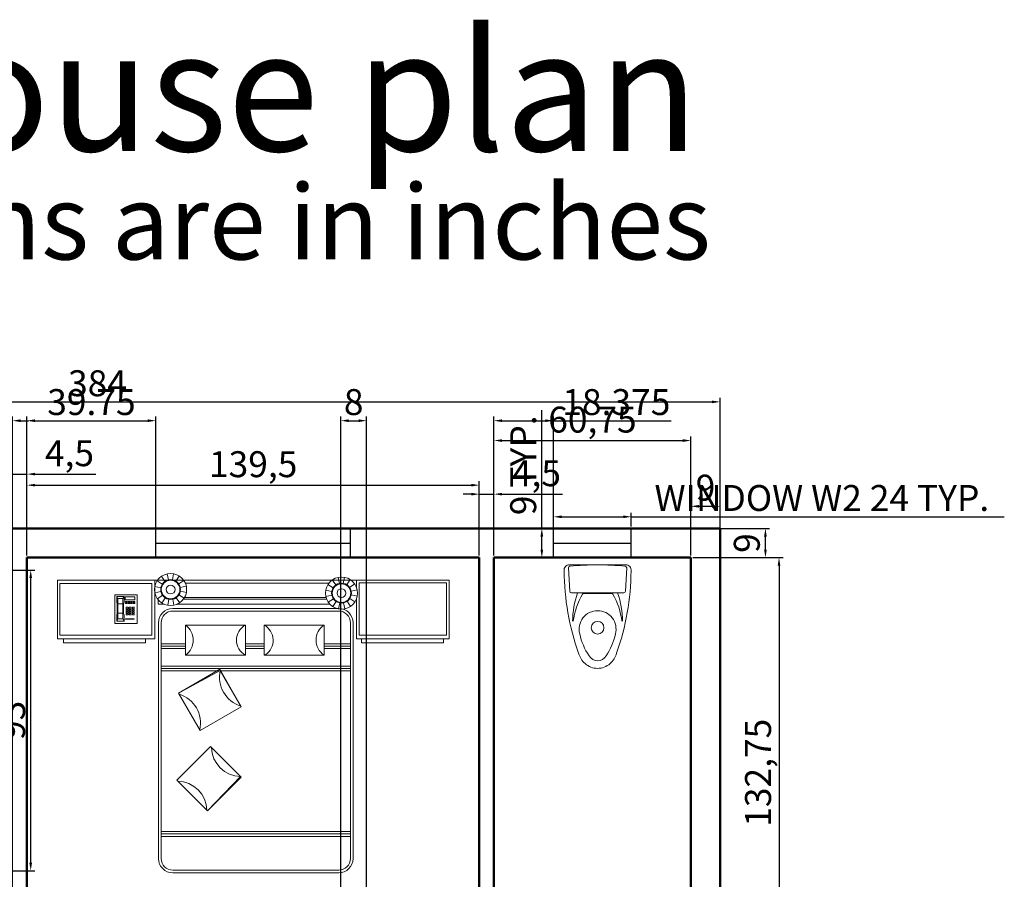
# Model space of a CAD drawing. Units: inches. Extents: x -349 to 9053, y 635 to 6001.
# Tile 6 of 7: x 498 to 802, y 1018 to 1283. Entities that reach past the tile are written whole.
import ezdxf

# ---------------------------------------------------------------- set-up
doc = ezdxf.new("R2010")
doc.units = ezdxf.units.IN
for name, color, linetype, lineweight in [('A-ANNO-DIMS', 2, 'Continuous', 18), ('A-ANNO-TEXT', 7, 'Continuous', 25), ('A-FLOR-FIXT', 7, 'Continuous', 18), ('A-FURN', 8, 'Continuous', 18), ('A-GLAZ', 4, 'Continuous', 25), ('A-WALL', 7, 'Continuous', 50)]:
    doc.layers.add(name, color=color, linetype=linetype, lineweight=lineweight)
doc.styles.get("Standard").update_dxf_attribs({"font": 'arial.ttf'})
doc.dimstyles.new('ISO-25', dxfattribs={"dimtxt": 8, "dimasz": 2.5, "dimexe": 1.25, "dimexo": 0.625, "dimtad": 1, "dimtxsty": 'Standard', "dimcen": 2.5, "dimadec": 0, "dimazin": 0, "dimtfac": 1, "dimtmove": 0, "dimatfit": 3, "dimfxl": 1, "dimarcsym": 0})

# ---------------------------------------------------------------- blocks, each defined once
blk = doc.blocks.new('A$C18EB7ED0')
for p, q in [((0.7653, 2.1814), (0.7911, 2.1442)), ((0.8076, 2.1998), (0.8172, 2.1555)), ((0.8537, 2.2006), (0.8456, 2.1559)), ((0.8966, 2.1836), (0.8721, 2.1455)), ((2.0643, 2.1733), (2.0739, 2.129)), ((2.1105, 2.1741), (2.1024, 2.1295)), ((0, 2.1539), (2.8801, 2.1539)), ((0, 1.7209), (0, 2.1539)), ((0.0187, 2.129), (0.695, 2.129)), ((0.0187, 1.7489), (0.0187, 2.129)), ((0.695, 2.129), (0.695, 1.7489)), ((0.7156, 2.1539), (0.7156, 1.7209)), ((0.7162, 2.1054), (0.7608, 2.0973)), ((0.7332, 2.1483), (0.7713, 2.1237)), ((0.9298, 2.1515), (0.8925, 2.1257)), ((0.9481, 2.1092), (0.9038, 2.0996)), ((0.941, 2.1314), (1.9968, 2.1314)), ((1.9899, 2.1218), (2.028, 2.0973)), ((2.022, 2.155), (2.0478, 2.1177)), ((2.1534, 2.1571), (2.1288, 2.119)), ((2.1865, 2.1251), (2.1493, 2.0992)), ((2.1997, 2.1), (2.1997, 2.1539)), ((2.2184, 2.1337), (2.8624, 2.1337)), ((2.2184, 1.7489), (2.2184, 2.1337)), ((2.8624, 2.1337), (2.8624, 1.7489)), ((2.8801, 2.1539), (2.8801, 1.7209)), ((0.5857, 2.0461), (0.4227, 2.0461)), ((0.4227, 2.0461), (0.4227, 1.8353)), ((0.4366, 2.0335), (0.4439, 2.018)), ((0.4903, 2.0335), (0.4366, 2.0335)), ((0.4366, 2.0335), (0.4366, 1.9902)), ((0.4824, 2.018), (0.4903, 2.0335)), ((0.4903, 1.9902), (0.4903, 2.0338)), ((0.5706, 2.0307), (0.4996, 2.0307)), ((0.4996, 2.0307), (0.4996, 2.0082)), ((0.5706, 2.0082), (0.5706, 2.0307)), ((0.5857, 1.8353), (0.5857, 2.0461)), ((0.717, 2.0593), (0.7613, 2.0688)), ((0.7353, 2.0169), (0.7726, 2.0427)), ((0.9319, 2.0202), (0.8938, 2.0447)), ((0.9489, 2.0631), (0.9043, 2.0712)), ((1.973, 2.0789), (2.0176, 2.0708)), ((1.9737, 2.0328), (2.0181, 2.0424)), ((2.2049, 2.0827), (2.1606, 2.0731)), ((2.2056, 2.0366), (2.161, 2.0447)), ((0.4366, 1.9902), (0.4391, 1.9789)), ((0.4391, 1.9789), (0.4391, 1.9067)), ((0.4824, 2.018), (0.4439, 2.018)), ((0.4824, 2.018), (0.4439, 2.018)), ((0.4439, 2.018), (0.4439, 1.8697)), ((0.4824, 1.978), (0.4439, 1.978)), ((0.4824, 1.8697), (0.4824, 2.018)), ((0.4903, 1.9902), (0.4871, 1.9789)), ((0.4871, 1.9789), (0.4871, 1.908)), ((0.4996, 2.0082), (0.5706, 2.0082)), ((0.514, 1.9963), (0.5013, 1.9963)), ((0.5013, 1.9963), (0.5013, 1.992)), ((0.5013, 1.992), (0.514, 1.992)), ((0.514, 1.9864), (0.5013, 1.9864)), ((0.5013, 1.9864), (0.5013, 1.9821)), ((0.5013, 1.9821), (0.514, 1.9821)), ((0.514, 1.992), (0.514, 1.9963)), ((0.514, 1.9821), (0.514, 1.9864)), ((0.5324, 1.9963), (0.5196, 1.9963)), ((0.5196, 1.9963), (0.5196, 1.992)), ((0.5196, 1.992), (0.5324, 1.992)), ((0.5324, 1.9864), (0.5196, 1.9864)), ((0.5196, 1.9864), (0.5196, 1.9821)), ((0.5196, 1.9821), (0.5324, 1.9821)), ((0.5324, 1.992), (0.5324, 1.9963)), ((0.5324, 1.9821), (0.5324, 1.9864)), ((0.5507, 1.9963), (0.538, 1.9963)), ((0.538, 1.9963), (0.538, 1.992)), ((0.538, 1.992), (0.5507, 1.992)), ((0.5507, 1.9864), (0.538, 1.9864)), ((0.538, 1.9864), (0.538, 1.9821)), ((0.538, 1.9821), (0.5507, 1.9821)), ((0.5507, 1.992), (0.5507, 1.9963)), ((0.5507, 1.9821), (0.5507, 1.9864)), ((0.5691, 1.9963), (0.5564, 1.9963)), ((0.5564, 1.9963), (0.5564, 1.992)), ((0.5564, 1.992), (0.5691, 1.992)), ((0.5691, 1.9864), (0.5564, 1.9864)), ((0.5564, 1.9864), (0.5564, 1.9821)), ((0.5564, 1.9821), (0.5691, 1.9821)), ((0.5691, 1.992), (0.5691, 1.9963)), ((0.5691, 1.9821), (0.5691, 1.9864)), ((0.7411, 2.0132), (0.7411, 1.9754)), ((0.7411, 1.9754), (0.7863, 1.9754)), ((0.7685, 1.9849), (0.7931, 2.023)), ((0.8114, 1.9679), (0.8195, 2.0125)), ((0.8575, 1.9687), (0.848, 2.013)), ((0.8999, 1.987), (0.8741, 2.0243)), ((0.8788, 1.9754), (2.0045, 1.9754)), ((1.9798, 2.0132), (0.9271, 2.0132)), ((1.9752, 2.0268), (0.9359, 2.0268)), ((1.9921, 1.9905), (2.0294, 2.0163)), ((2.0252, 1.9584), (2.0498, 1.9965)), ((2.0682, 1.9414), (2.0763, 1.986)), ((2.1143, 1.9422), (2.1047, 1.9865)), ((2.1566, 1.9605), (2.1308, 1.9978)), ((2.1887, 1.9937), (2.1506, 2.0183)), ((2.1742, 1.9754), (2.1771, 1.9754)), ((2.1771, 1.9754), (2.1771, 1.9785)), ((2.1997, 1.7209), (2.1997, 2.0155)), ((0.4391, 1.9067), (0.4366, 1.8971)), ((0.4366, 1.8971), (0.4366, 1.8504)), ((0.4439, 1.9101), (0.4824, 1.9101)), ((0.4871, 1.908), (0.4903, 1.8971)), ((0.4903, 1.8499), (0.4903, 1.8971)), ((0.52, 1.9534), (0.5062, 1.9534)), ((0.5062, 1.9534), (0.5062, 1.9417)), ((0.5062, 1.9417), (0.52, 1.9417)), ((0.52, 1.9385), (0.5062, 1.9385)), ((0.5062, 1.9385), (0.5062, 1.9269)), ((0.5062, 1.9269), (0.52, 1.9269)), ((0.52, 1.9237), (0.5062, 1.9237)), ((0.5062, 1.9237), (0.5062, 1.9121)), ((0.5062, 1.9121), (0.52, 1.9121)), ((0.52, 1.9089), (0.5062, 1.9089)), ((0.5062, 1.9089), (0.5062, 1.8972)), ((0.5062, 1.8972), (0.52, 1.8972)), ((0.52, 1.9417), (0.52, 1.9534)), ((0.52, 1.9269), (0.52, 1.9385)), ((0.52, 1.9121), (0.52, 1.9237)), ((0.52, 1.8972), (0.52, 1.9089)), ((0.5426, 1.9534), (0.5288, 1.9534)), ((0.5288, 1.9534), (0.5288, 1.9417)), ((0.5288, 1.9417), (0.5426, 1.9417)), ((0.5426, 1.9385), (0.5288, 1.9385)), ((0.5288, 1.9385), (0.5288, 1.9269)), ((0.5288, 1.9269), (0.5426, 1.9269)), ((0.5426, 1.9237), (0.5288, 1.9237)), ((0.5288, 1.9237), (0.5288, 1.9121)), ((0.5288, 1.9121), (0.5426, 1.9121)), ((0.5426, 1.9089), (0.5288, 1.9089)), ((0.5288, 1.9089), (0.5288, 1.8972)), ((0.5288, 1.8972), (0.5426, 1.8972)), ((0.5426, 1.9417), (0.5426, 1.9534)), ((0.5426, 1.9269), (0.5426, 1.9385)), ((0.5426, 1.9121), (0.5426, 1.9237)), ((0.5426, 1.8972), (0.5426, 1.9089)), ((0.5659, 1.9534), (0.5521, 1.9534)), ((0.5521, 1.9534), (0.5521, 1.9417)), ((0.5521, 1.9417), (0.5659, 1.9417)), ((0.5659, 1.9385), (0.5521, 1.9385)), ((0.5521, 1.9385), (0.5521, 1.9269)), ((0.5521, 1.9269), (0.5659, 1.9269)), ((0.5659, 1.9237), (0.5521, 1.9237)), ((0.5521, 1.9237), (0.5521, 1.9121)), ((0.5521, 1.9121), (0.5659, 1.9121)), ((0.5659, 1.9089), (0.5521, 1.9089)), ((0.5521, 1.9089), (0.5521, 1.8972)), ((0.5521, 1.8972), (0.5659, 1.8972)), ((0.5659, 1.9417), (0.5659, 1.9534)), ((0.5659, 1.9269), (0.5659, 1.9385)), ((0.5659, 1.9121), (0.5659, 1.9237)), ((0.5659, 1.8972), (0.5659, 1.9089)), ((2.0691, 1.9452), (0.8491, 1.9452)), ((2.0691, 1.926), (0.8491, 1.926)), ((0.4227, 1.8353), (0.5857, 1.8353)), ((0.4439, 1.8697), (0.4366, 1.8504)), ((0.4366, 1.8504), (0.4903, 1.8504)), ((0.4824, 1.8697), (0.4439, 1.8697)), ((0.4439, 1.8697), (0.4824, 1.8697)), ((0.4903, 1.8504), (0.4824, 1.8697)), ((0.5208, 1.8697), (0.5009, 1.8697)), ((0.5009, 1.8697), (0.5009, 1.8657)), ((0.5009, 1.8657), (0.5208, 1.8657)), ((0.5208, 1.8657), (0.5208, 1.8697)), ((0.5433, 1.8697), (0.5234, 1.8697)), ((0.5234, 1.8697), (0.5234, 1.8657)), ((0.5234, 1.8657), (0.5433, 1.8657)), ((0.5433, 1.8657), (0.5433, 1.8697)), ((0.5658, 1.8697), (0.546, 1.8697)), ((0.546, 1.8697), (0.546, 1.8657)), ((0.546, 1.8657), (0.5658, 1.8657)), ((0.5658, 1.8657), (0.5658, 1.8697)), ((0.7439, 1.8401), (0.7439, 0.1052)), ((0.7632, 1.8401), (0.7632, 0.1052)), ((0.9429, 1.8231), (1.3829, 1.8231)), ((0.9429, 1.601), (0.9429, 1.8231)), ((1.3829, 1.8231), (1.3829, 1.601)), ((1.5207, 1.601), (1.5207, 1.8231)), ((1.5207, 1.8231), (1.9608, 1.8231)), ((1.9608, 1.8231), (1.9608, 1.601)), ((2.155, 0.1052), (2.155, 1.8401)), ((2.1743, 0.1052), (2.1743, 1.8401)), ((0.695, 1.7489), (0.0187, 1.7489)), ((2.8624, 1.7489), (2.2184, 1.7489)), ((0.7156, 1.7209), (0, 1.7209)), ((0, 1.7209), (0.6483, 1.7209)), ((0.0462, 1.6929), (0.0462, 1.7209)), ((0.6483, 1.6929), (0.0462, 1.6929)), ((0.6483, 1.7209), (0.6483, 1.6929)), ((0.7632, 1.6858), (0.9429, 1.6858)), ((0.7632, 1.6678), (0.9429, 1.6678)), ((1.3829, 1.6858), (1.5207, 1.6858)), ((1.3829, 1.6678), (1.5207, 1.6678)), ((1.9608, 1.6858), (2.155, 1.6858)), ((1.9608, 1.6678), (2.155, 1.6678)), ((2.8801, 1.7209), (2.1997, 1.7209)), ((2.2369, 1.7209), (2.8801, 1.7209)), ((2.2369, 1.6929), (2.2369, 1.7209)), ((2.839, 1.6929), (2.2369, 1.6929)), ((2.839, 1.7209), (2.839, 1.6929)), ((0.7632, 1.6498), (0.9429, 1.6498)), ((1.3829, 1.601), (0.9429, 1.601)), ((1.3829, 1.6498), (1.5207, 1.6498)), ((1.9608, 1.601), (1.5207, 1.601)), ((1.9608, 1.6498), (2.155, 1.6498)), ((0.7632, 1.5215), (2.155, 1.5215)), ((0.7632, 1.5035), (2.155, 1.5035)), ((0.7632, 1.4855), (2.155, 1.4855)), ((0.8904, 1.3226), (1.1935, 1.4976)), ((0.8904, 1.3226), (1.1982, 1.4894)), ((1.1935, 1.4976), (1.3524, 1.2224)), ((1.1982, 1.4894), (1.3524, 1.2224)), ((1.0493, 1.0474), (0.8904, 1.3226)), ((1.0493, 1.0474), (0.8904, 1.3226)), ((1.3524, 1.2224), (1.0493, 1.0474)), ((1.3524, 1.2224), (1.0493, 1.0474)), ((0.8789, 0.6811), (1.1264, 0.9286)), ((0.8789, 0.6811), (1.1264, 0.9286)), ((1.1264, 0.9286), (1.3473, 0.7077)), ((1.1264, 0.9286), (1.3511, 0.7039)), ((1.1036, 0.4564), (0.8789, 0.6811)), ((1.1036, 0.4564), (0.8789, 0.6811)), ((1.3473, 0.7077), (1.1036, 0.4564)), ((1.3511, 0.7039), (1.1036, 0.4564)), ((0.7632, 0.3045), (2.155, 0.3045)), ((0.7632, 0.2865), (2.155, 0.2865)), ((0.7632, 0.2685), (2.155, 0.2685)), ((0.8491, 0.0193), (2.0691, 0.0193)), ((0.8491, 0), (2.0691, 0))]:
    blk.add_line(p, q)
for centre, radius in [((0.8326, 2.0842), 0.1182), ((2.0893, 2.0578), 0.1182), ((0.8326, 2.0842), 0.0729), ((0.8326, 2.0842), 0.0684), ((0.8326, 2.0842), 0.0328), ((2.0893, 2.0578), 0.0729), ((2.0893, 2.0578), 0.0684), ((2.0893, 2.0578), 0.0328)]:
    blk.add_circle(centre, radius)
for centre, radius, start, end in [((0.8491, 1.8401), 0.1052, 90, 180), ((0.8491, 1.8401), 0.0859, 90, 180), ((2.0691, 1.8401), 0.1052, 0, 90), ((2.0691, 1.8401), 0.0859, 0, 90), ((0.8604, 1.712), 0.1383, 306.59595, 53.40405), ((1.4431, 1.712), 0.1263, 118.46186, 241.53814), ((1.4584, 1.7106), 0.1286, 303.40233, 61.02638), ((2.0371, 1.712), 0.1347, 124.50267, 235.49733), ((1.4126, 1.4383), 0.2204, 166.58792, 253.41208), ((0.8322, 1.1031), 0.2204, 346.58792, 73.41208), ((1.3534, 0.928), 0.2204, 181.58792, 268.41208), ((0.8795, 0.4541), 0.2204, 1.58792, 88.41208), ((0.8491, 0.1052), 0.1052, 180, 270), ((0.8491, 0.1052), 0.0859, 180, 270), ((2.0691, 0.1052), 0.1052, 270, 0), ((2.0691, 0.1052), 0.0859, 270, 0)]:
    blk.add_arc(centre, radius, start, end)
blk = doc.blocks.new('A$C444A5E9C')
at = {"ltscale": 20}
for p, q in [((0.0411, 0.5655), (0.0321, 0.7371)), ((0.2458, 0.76), (0.0398, 0.76)), ((0.0536, 0.5537), (0.2458, 0.5537)), ((0.141, 0.5487), (0.2458, 0.5487))]:
    blk.add_line(p, q, dxfattribs=at)
for p, q in [((0.2458, 0.76), (0.4517, 0.76)), ((0.4504, 0.5655), (0.4594, 0.7371)), ((0.4379, 0.5537), (0.2458, 0.5537)), ((0.3505, 0.5487), (0.2458, 0.5487))]:
    blk.add_line(p, q)
blk.add_circle((0.2458, 0.2982), 0.0465, dxfattribs=at)
for centre, radius, start, end in [((0.0398, 0.72), 0.04, 90, 185.821), ((0.0441, 0.7377), 0.012, 95.84387, 183), ((0.2455, -1.2297), 1.9897, 89.99241, 95.84387), ((1.8697, 0.7335), 1.8698, 180.53729, 199.44062), ((0.0536, 0.5662), 0.0125, 183, 270), ((0.7661, 0.3277), 0.7045, 161.29061, 178.53633), ((0.58, 0.2848), 0.5159, 149.71646, 173.22437), ((0.141, 0.5412), 0.0075, 90, 149.71646), ((0.2463, 0.2875), 0.1361, 90.23685, 194.54903), ((0.2452, 0.2875), 0.1361, 345.45097, 89.76315), ((0.561, 0.3494), 0.4566, 192.1399, 214.27057), ((-0.0695, 0.3494), 0.4566, 325.72943, 347.8601), ((0.2665, 0.1585), 0.1669, 196.47232, 227.66237), ((0.2465, 0.1287), 0.0727, 210.08399, 269.41891), ((0.245, 0.1287), 0.0727, 270.58109, 329.91601), ((0.2458, 0.137), 0.137, 228.04012, 270)]:
    blk.add_arc(centre, radius, start, end, dxfattribs=at)
for centre, radius, start, end in [((0.246, -1.2297), 1.9897, 84.15613, 90.00759), ((0.4474, 0.7377), 0.012, 357, 84.15613), ((0.4517, 0.72), 0.04, 354.179, 90), ((-1.3782, 0.7335), 1.8698, 340.55938, 359.46271), ((0.3505, 0.5412), 0.0075, 30.28354, 90), ((-0.0885, 0.2848), 0.5159, 6.77563, 30.28354), ((-0.2746, 0.3277), 0.7045, 1.46367, 18.70939), ((0.4379, 0.5662), 0.0125, 270, 357), ((0.225, 0.1585), 0.1669, 312.33763, 343.52768), ((0.2458, 0.137), 0.137, 270, 311.95988)]:
    blk.add_arc(centre, radius, start, end)
blk = doc.blocks.new('*D7')
at = {"layer": 'A-ANNO-DIMS', "color": 0, "lineweight": -2, "transparency": 16777216}
for p, q in [((705.63, 1126), (729.24, 1126)), ((727.99, 1119.5), (727.99, 1123.5)), ((705.63, 1117), (729.24, 1117))]:
    blk.add_line(p, q, dxfattribs=at)
at = {"layer": 'A-ANNO-DIMS', "color": 0, "transparency": 16777216}
for points in [[(727.57, 1123.5), (728.4, 1123.5), (727.99, 1126)], [(727.57, 1119.5), (728.4, 1119.5), (727.99, 1117)]]:
    blk.add_solid(points, dxfattribs=at)
at = {"layer": 'Defpoints', "color": 0, "transparency": 16777216}
for p in [(705, 1126), (727.99, 1126), (705, 1117)]:
    blk.add_point(p, dxfattribs=at)
at = {"layer": 'A-ANNO-DIMS', "color": 0, "transparency": 16777216, "insert": (723.28, 1121.5), "char_height": 8, "attachment_point": 5, "rotation": 90}
blk.add_mtext('9', dxfattribs=at)
blk = doc.blocks.new('*D14')
at = {"layer": 'A-ANNO-DIMS', "color": 0, "lineweight": -2, "transparency": 16777216}
for p, q in [((493.25, 1142.76), (490.75, 1142.76)), ((495.75, 1117.62), (495.75, 1144.01)), ((495.75, 1142.76), (500.25, 1142.76)), ((500.25, 1117.62), (500.25, 1144.01)), ((502.75, 1142.76), (521.45, 1142.76))]:
    blk.add_line(p, q, dxfattribs=at)
at = {"layer": 'A-ANNO-DIMS', "color": 0, "transparency": 16777216}
for points in [[(493.25, 1143.18), (493.25, 1142.35), (495.75, 1142.76)], [(502.75, 1143.18), (502.75, 1142.35), (500.25, 1142.76)]]:
    blk.add_solid(points, dxfattribs=at)
at = {"layer": 'Defpoints', "color": 0, "transparency": 16777216}
for p in [(500.25, 1142.76), (495.75, 1117), (500.25, 1117)]:
    blk.add_point(p, dxfattribs=at)
at = {"layer": 'A-ANNO-DIMS', "color": 0, "transparency": 16777216, "insert": (513.35, 1148.18), "char_height": 8, "attachment_point": 5}
blk.add_mtext('4,5', dxfattribs=at)
blk = doc.blocks.new('*D15')
at = {"layer": 'A-ANNO-DIMS', "color": 0, "lineweight": -2, "transparency": 16777216}
for p, q in [((500.25, 1117.62), (500.25, 1140.61)), ((502.75, 1139.36), (637.25, 1139.36)), ((639.75, 1117.62), (639.75, 1140.61))]:
    blk.add_line(p, q, dxfattribs=at)
at = {"layer": 'A-ANNO-DIMS', "color": 0, "transparency": 16777216}
for points in [[(502.75, 1139.78), (502.75, 1138.94), (500.25, 1139.36)], [(637.25, 1139.78), (637.25, 1138.94), (639.75, 1139.36)]]:
    blk.add_solid(points, dxfattribs=at)
at = {"layer": 'Defpoints', "color": 0, "transparency": 16777216}
for p in [(639.75, 1139.36), (500.25, 1117), (639.75, 1117)]:
    blk.add_point(p, dxfattribs=at)
at = {"layer": 'A-ANNO-DIMS', "color": 0, "transparency": 16777216, "insert": (570, 1144.79), "char_height": 8, "attachment_point": 5}
blk.add_mtext('139,5', dxfattribs=at)
blk = doc.blocks.new('*D16')
at = {"layer": 'A-ANNO-DIMS', "color": 0, "lineweight": -2, "transparency": 16777216}
for p, q in [((637.25, 1136.58), (634.75, 1136.58)), ((639.75, 1117.62), (639.75, 1137.83)), ((639.75, 1136.58), (644.25, 1136.58)), ((644.25, 1117.62), (644.25, 1137.83)), ((646.75, 1136.58), (665.45, 1136.58))]:
    blk.add_line(p, q, dxfattribs=at)
at = {"layer": 'A-ANNO-DIMS', "color": 0, "transparency": 16777216}
for points in [[(637.25, 1137), (637.25, 1136.17), (639.75, 1136.58)], [(646.75, 1137), (646.75, 1136.17), (644.25, 1136.58)]]:
    blk.add_solid(points, dxfattribs=at)
at = {"layer": 'Defpoints', "color": 0, "transparency": 16777216}
for p in [(644.25, 1136.58), (639.75, 1117), (644.25, 1117)]:
    blk.add_point(p, dxfattribs=at)
at = {"layer": 'A-ANNO-DIMS', "color": 0, "transparency": 16777216, "insert": (657.35, 1142), "char_height": 8, "attachment_point": 5}
blk.add_mtext('4,5', dxfattribs=at)
blk = doc.blocks.new('*D17')
at = {"layer": 'A-ANNO-DIMS', "color": 0, "lineweight": -2, "transparency": 16777216}
for p, q in [((644.25, 1117.62), (644.25, 1154.37)), ((705, 1117.62), (705, 1154.37)), ((646.75, 1153.12), (702.5, 1153.12))]:
    blk.add_line(p, q, dxfattribs=at)
at = {"layer": 'A-ANNO-DIMS', "color": 0, "transparency": 16777216}
for points in [[(646.75, 1153.54), (646.75, 1152.7), (644.25, 1153.12)], [(702.5, 1153.54), (702.5, 1152.7), (705, 1153.12)]]:
    blk.add_solid(points, dxfattribs=at)
at = {"layer": 'Defpoints', "color": 0, "transparency": 16777216}
for p in [(705, 1153.12), (644.25, 1117), (705, 1117)]:
    blk.add_point(p, dxfattribs=at)
at = {"layer": 'A-ANNO-DIMS', "color": 0, "transparency": 16777216, "insert": (674.62, 1158.55), "char_height": 8, "attachment_point": 5}
blk.add_mtext('60,75', dxfattribs=at)
blk = doc.blocks.new('*D18')
at = {"layer": 'A-ANNO-DIMS', "color": 0, "lineweight": -2, "transparency": 16777216}
for p, q in [((705, 1117.62), (705, 1134.09)), ((707.5, 1132.84), (711.5, 1132.84)), ((714, 1117.62), (714, 1134.09))]:
    blk.add_line(p, q, dxfattribs=at)
at = {"layer": 'A-ANNO-DIMS', "color": 0, "transparency": 16777216}
for points in [[(707.5, 1133.26), (707.5, 1132.42), (705, 1132.84)], [(711.5, 1133.26), (711.5, 1132.42), (714, 1132.84)]]:
    blk.add_solid(points, dxfattribs=at)
at = {"layer": 'Defpoints', "color": 0, "transparency": 16777216}
for p in [(714, 1132.84), (705, 1117), (714, 1117)]:
    blk.add_point(p, dxfattribs=at)
at = {"layer": 'A-ANNO-DIMS', "color": 0, "transparency": 16777216, "insert": (709.5, 1137.55), "char_height": 8, "attachment_point": 5}
blk.add_mtext('9', dxfattribs=at)
blk = doc.blocks.new('*D19')
at = {"layer": 'A-ANNO-DIMS', "color": 0, "lineweight": -2, "transparency": 16777216}
for p, q in [((330, 1126.62), (330, 1166.31)), ((714, 1126.62), (714, 1166.31)), ((332.5, 1165.06), (711.5, 1165.06))]:
    blk.add_line(p, q, dxfattribs=at)
at = {"layer": 'A-ANNO-DIMS', "color": 0, "transparency": 16777216}
for points in [[(332.5, 1165.47), (332.5, 1164.64), (330, 1165.06)], [(711.5, 1165.47), (711.5, 1164.64), (714, 1165.06)]]:
    blk.add_solid(points, dxfattribs=at)
at = {"layer": 'Defpoints', "color": 0, "transparency": 16777216}
for p in [(714, 1165.06), (330, 1126), (714, 1126)]:
    blk.add_point(p, dxfattribs=at)
at = {"layer": 'A-ANNO-DIMS', "color": 0, "transparency": 16777216, "insert": (522, 1169.77), "char_height": 8, "attachment_point": 5}
blk.add_mtext('384', dxfattribs=at)
blk = doc.blocks.new('*D32')
at = {"layer": 'A-ANNO-DIMS', "color": 0, "lineweight": -2, "transparency": 16777216}
for p, q in [((705.63, 1117), (733.43, 1117)), ((732.18, 1114.5), (732.18, 986.75)), ((705.63, 984.25), (733.43, 984.25))]:
    blk.add_line(p, q, dxfattribs=at)
at = {"layer": 'A-ANNO-DIMS', "color": 0, "transparency": 16777216}
for points in [[(731.76, 1114.5), (732.59, 1114.5), (732.18, 1117)], [(731.76, 986.75), (732.59, 986.75), (732.18, 984.25)]]:
    blk.add_solid(points, dxfattribs=at)
at = {"layer": 'Defpoints', "color": 0, "transparency": 16777216}
for p in [(705, 1117), (705, 984.25), (732.18, 984.25)]:
    blk.add_point(p, dxfattribs=at)
at = {"layer": 'A-ANNO-DIMS', "color": 0, "transparency": 16777216, "insert": (726.74, 1050.62), "char_height": 8, "attachment_point": 5, "rotation": 90}
blk.add_mtext('132,75', dxfattribs=at)
blk = doc.blocks.new('WIN-60IN')
for p, q in [((0, -4.5), (0, 4.5)), ((60, -4.5), (60, 4.5)), ((0, 0), (60, 0))]:
    blk.add_line(p, q)
blk = doc.blocks.new('WIN-24IN')
for p, q in [((0, -4.5), (0, 4.5)), ((24, -4.5), (24, 4.5)), ((0, 0), (24, 0))]:
    blk.add_line(p, q)
blk = doc.blocks.new('*D47')
at = {"layer": 'A-ANNO-DIMS', "color": 0, "lineweight": -2, "transparency": 16777216}
for p, q in [((662.62, 1126.62), (662.62, 1130.85)), ((665.12, 1129.6), (684.12, 1129.6)), ((686.62, 1126.62), (686.62, 1130.85)), ((686.62, 1129.6), (801.65, 1129.6))]:
    blk.add_line(p, q, dxfattribs=at)
at = {"layer": 'A-ANNO-DIMS', "color": 0, "transparency": 16777216}
for points in [[(665.12, 1130.02), (665.12, 1129.18), (662.62, 1129.6)], [(684.12, 1130.02), (684.12, 1129.18), (686.62, 1129.6)]]:
    blk.add_solid(points, dxfattribs=at)
at = {"layer": 'Defpoints', "color": 0, "transparency": 16777216}
for p in [(686.62, 1129.6), (662.62, 1126), (686.62, 1126)]:
    blk.add_point(p, dxfattribs=at)
at = {"layer": 'A-ANNO-DIMS', "color": 0, "transparency": 16777216, "insert": (745.39, 1134.36), "char_height": 8, "attachment_point": 5}
blk.add_mtext('WINDOW W2 24 TYP.', dxfattribs=at)
blk = doc.blocks.new('*D48')
at = {"layer": 'A-ANNO-DIMS', "color": 0, "lineweight": -2, "transparency": 16777216}
for p, q in [((659.03, 1126), (659.03, 1162.48)), ((662, 1126), (657.78, 1126)), ((659.03, 1119.5), (659.03, 1123.5)), ((662, 1117), (657.78, 1117))]:
    blk.add_line(p, q, dxfattribs=at)
at = {"layer": 'A-ANNO-DIMS', "color": 0, "transparency": 16777216}
for points in [[(658.61, 1123.5), (659.44, 1123.5), (659.03, 1126)], [(658.61, 1119.5), (659.44, 1119.5), (659.03, 1117)]]:
    blk.add_solid(points, dxfattribs=at)
at = {"layer": 'Defpoints', "color": 0, "transparency": 16777216}
for p in [(659.03, 1126), (662.63, 1126), (662.63, 1117)]:
    blk.add_point(p, dxfattribs=at)
at = {"layer": 'A-ANNO-DIMS', "color": 0, "transparency": 16777216, "insert": (654.32, 1145.49), "char_height": 8, "attachment_point": 5, "rotation": 90}
blk.add_mtext('9 TYP.', dxfattribs=at)
blk = doc.blocks.new('*D54')
at = {"layer": 'A-ANNO-DIMS', "color": 0, "lineweight": -2, "transparency": 16777216}
for p, q in [((482.52, 1113.17), (502.65, 1113.17)), ((501.4, 1022.89), (501.4, 1110.67)), ((482.52, 1020.39), (502.65, 1020.39))]:
    blk.add_line(p, q, dxfattribs=at)
at = {"layer": 'A-ANNO-DIMS', "color": 0, "transparency": 16777216}
for points in [[(500.98, 1110.67), (501.82, 1110.67), (501.4, 1113.17)], [(500.98, 1022.89), (501.82, 1022.89), (501.4, 1020.39)]]:
    blk.add_solid(points, dxfattribs=at)
at = {"layer": 'Defpoints', "color": 0, "transparency": 16777216}
for p in [(481.9, 1113.17), (501.4, 1113.17), (481.9, 1020.39)]:
    blk.add_point(p, dxfattribs=at)
at = {"layer": 'A-ANNO-DIMS', "color": 0, "transparency": 16777216, "insert": (496.69, 1066.78), "char_height": 8, "attachment_point": 5, "rotation": 90}
blk.add_mtext('93', dxfattribs=at)
blk = doc.blocks.new('*D68')
at = {"layer": 'A-ANNO-DIMS', "color": 0, "lineweight": -2, "transparency": 16777216}
for p, q in [((597, 794.38), (597, 1160.5)), ((605, 794.38), (605, 1160.5)), ((599.5, 1159.25), (602.5, 1159.25))]:
    blk.add_line(p, q, dxfattribs=at)
at = {"layer": 'A-ANNO-DIMS', "color": 0, "transparency": 16777216}
for points in [[(599.5, 1159.67), (599.5, 1158.83), (597, 1159.25)], [(602.5, 1159.67), (602.5, 1158.83), (605, 1159.25)]]:
    blk.add_solid(points, dxfattribs=at)
at = {"layer": 'Defpoints', "color": 0, "transparency": 16777216}
for p in [(605, 1159.25), (597, 793.75), (605, 793.75)]:
    blk.add_point(p, dxfattribs=at)
at = {"layer": 'A-ANNO-DIMS', "color": 0, "transparency": 16777216, "insert": (601, 1163.96), "char_height": 8, "attachment_point": 5}
blk.add_mtext('8', dxfattribs=at)
blk = doc.blocks.new('*D70')
at = {"layer": 'A-ANNO-DIMS', "color": 0, "lineweight": -2, "transparency": 16777216}
for p, q in [((500.25, 1117.62), (500.25, 1160.5)), ((540, 1117.62), (540, 1160.5)), ((502.75, 1159.25), (537.5, 1159.25))]:
    blk.add_line(p, q, dxfattribs=at)
at = {"layer": 'A-ANNO-DIMS', "color": 0, "transparency": 16777216}
for points in [[(502.75, 1159.67), (502.75, 1158.83), (500.25, 1159.25)], [(537.5, 1159.67), (537.5, 1158.83), (540, 1159.25)]]:
    blk.add_solid(points, dxfattribs=at)
at = {"layer": 'Defpoints', "color": 0, "transparency": 16777216}
for p in [(540, 1159.25), (500.25, 1117), (540, 1117)]:
    blk.add_point(p, dxfattribs=at)
at = {"layer": 'A-ANNO-DIMS', "color": 0, "transparency": 16777216, "insert": (520.12, 1163.96), "char_height": 8, "attachment_point": 5}
blk.add_mtext('39.75', dxfattribs=at)
blk = doc.blocks.new('*D71')
at = {"layer": 'A-ANNO-DIMS', "color": 0, "lineweight": -2, "transparency": 16777216}
for p, q in [((644.25, 1117.62), (644.25, 1160.5)), ((662.62, 1117.62), (662.62, 1160.5)), ((646.75, 1159.25), (660.12, 1159.25)), ((662.62, 1159.25), (698.89, 1159.25))]:
    blk.add_line(p, q, dxfattribs=at)
at = {"layer": 'A-ANNO-DIMS', "color": 0, "transparency": 16777216}
for points in [[(646.75, 1159.67), (646.75, 1158.83), (644.25, 1159.25)], [(660.12, 1159.67), (660.12, 1158.83), (662.62, 1159.25)]]:
    blk.add_solid(points, dxfattribs=at)
at = {"layer": 'Defpoints', "color": 0, "transparency": 16777216}
for p in [(662.62, 1159.25), (644.25, 1117), (662.62, 1117)]:
    blk.add_point(p, dxfattribs=at)
at = {"layer": 'A-ANNO-DIMS', "color": 0, "transparency": 16777216, "insert": (682.01, 1163.96), "char_height": 8, "attachment_point": 5}
blk.add_mtext('18.375', dxfattribs=at)
blk = doc.blocks.new('*D76')
at = {"layer": 'A-ANNO-DIMS', "color": 0, "lineweight": -2, "transparency": 16777216}
for p, q in [((491.75, 878.37), (491.75, 1160.5)), ((495.75, 878.37), (495.75, 1160.5)), ((489.25, 1159.25), (479.97, 1159.25)), ((495.75, 1159.25), (491.75, 1159.25)), ((498.25, 1159.25), (500.75, 1159.25))]:
    blk.add_line(p, q, dxfattribs=at)
at = {"layer": 'A-ANNO-DIMS', "color": 0, "transparency": 16777216}
for points in [[(489.25, 1159.67), (489.25, 1158.83), (491.75, 1159.25)], [(498.25, 1159.67), (498.25, 1158.83), (495.75, 1159.25)]]:
    blk.add_solid(points, dxfattribs=at)
at = {"layer": 'Defpoints', "color": 0, "transparency": 16777216}
for p in [(491.75, 1159.25), (491.75, 877.75), (495.75, 877.75)]:
    blk.add_point(p, dxfattribs=at)
at = {"layer": 'A-ANNO-DIMS', "color": 0, "transparency": 16777216, "insert": (483.36, 1163.88), "char_height": 8, "attachment_point": 5}
blk.add_mtext('4', dxfattribs=at)

msp = doc.modelspace()

# ---------------------------------------------------------------- linework, layer by layer
at = {"layer": 'A-WALL'}
for p, q in [((714, 1126), (330, 1126)), ((714, 670), (714, 1126)), ((500.25, 1117), (500.25, 984.25)), ((500.25, 1117), (639.75, 1117)), ((639.75, 1117), (500.25, 1117)), ((639.75, 1117), (639.75, 984.25)), ((705, 1117), (644.25, 1117)), ((644.25, 1117), (644.25, 984.25)), ((644.25, 1117), (705, 1117)), ((705, 984.25), (705, 1117))]:
    msp.add_line(p, q, dxfattribs=at)

# ---------------------------------------------------------------- block references
at = {"layer": 'A-FLOR-FIXT', "xscale": 42.04428802120991, "yscale": 42.04428802120991, "zscale": 42.04428802120991}
msp.add_blockref('A$C444A5E9C', (665.8881, 1082.827), dxfattribs=at)
at = {"layer": 'A-FURN', "xscale": 41.93766115492463, "yscale": 41.93766115492463, "zscale": 41.93766115492463}
msp.add_blockref('A$C18EB7ED0', (509.6195, 1019.7498), dxfattribs=at)
at = {"layer": 'A-GLAZ'}
for name, p in [('WIN-60IN', (540, 1121.5)), ('WIN-24IN', (662.625, 1121.5))]:
    msp.add_blockref(name, p, dxfattribs=at)

# ---------------------------------------------------------------- texts
at = {"layer": 'A-ANNO-TEXT'}
for s, height, p in [('3bhk house plan', 37.335229, (315.2717, 1242.4307)), ('all dimensions are in inches', 23.100038, (306.0951, 1208.9899))]:
    msp.add_text(s, height=height, dxfattribs=at).set_placement(p)

# ---------------------------------------------------------------- dimensions: what is measured, and where the dimension line sits
at = {"layer": 'A-ANNO-DIMS'}
for base, p1, p2, override, picture, middle in [((714, 1165.0562), (330, 1126), (714, 1126), {"dimclrd": 0, "dimclre": 0, "dimclrt": 0}, '*D19', (522, 1169.7685)), ((491.75, 1159.25), (495.75, 877.75), (491.75, 877.75), {"dimdec": 0, "dimlfac": 1, "dimrnd": 0, "dimzin": 0, "dimdsep": 46, "dimlunit": 2}, '*D76', (483.3583, 1163.875)), ((540, 1159.25), (500.25, 1117), (540, 1117), {"dimdec": 2, "dimlfac": 1, "dimrnd": 0, "dimzin": 0, "dimdsep": 46, "dimlunit": 2}, '*D70', (520.125, 1163.9623)), ((605, 1159.25), (597, 793.75), (605, 793.75), {"dimdec": 0, "dimlfac": 1, "dimrnd": 0, "dimzin": 0, "dimdsep": 46, "dimlunit": 2}, '*D68', (601, 1163.9596)), ((662.625, 1159.25), (644.25, 1117), (662.625, 1117), {"dimdec": 3, "dimlfac": 1, "dimrnd": 0, "dimzin": 0, "dimdsep": 46, "dimlunit": 2}, '*D71', (682.0092, 1163.9623)), ((705, 1153.1216), (644.25, 1117), (705, 1117), {"dimclrd": 0, "dimclre": 0, "dimclrt": 0}, '*D17', (674.625, 1158.5542)), ((500.25, 1142.763), (495.75, 1117), (500.25, 1117), {"dimclrd": 0, "dimclre": 0, "dimclrt": 0}, '*D14', (513.3484, 1148.1793)), ((639.75, 1139.359), (500.25, 1117), (639.75, 1117), {"dimclrd": 0, "dimclre": 0, "dimclrt": 0}, '*D15', (570, 1144.7916)), ((644.25, 1136.5818), (639.75, 1117), (644.25, 1117), {"dimclrd": 0, "dimclre": 0, "dimclrt": 0}, '*D16', (657.3484, 1141.9981)), ((714, 1132.8402), (705, 1117), (714, 1117), {"dimclrd": 0, "dimclre": 0, "dimclrt": 0}, '*D18', (709.5, 1137.5498))]:
    dim = msp.add_linear_dim(base=base, p1=p1, p2=p2, dimstyle='ISO-25', override=override, dxfattribs=at)
    dim.commit()
    dim.dimension.update_dxf_attribs({"geometry": picture, "text_midpoint": middle})
dim = msp.add_linear_dim(base=(659.025, 1126), p1=(662.625, 1117), p2=(662.625, 1126), angle=90, text='<> TYP.', dimstyle='ISO-25', override={"dimdec": 0, "dimlfac": 1, "dimrnd": 0, "dimzin": 0, "dimdsep": 46, "dimlunit": 2}, dxfattribs=at)
dim.commit()
dim.dimension.update_dxf_attribs({"geometry": '*D48', "text_midpoint": (654.3154, 1145.4879)})
dim = msp.add_linear_dim(base=(686.625, 1129.6), p1=(662.625, 1126), p2=(686.625, 1126), text='WINDOW W2 <> TYP.', dimstyle='ISO-25', override={"dimdec": 0, "dimlfac": 1, "dimrnd": 0, "dimzin": 0, "dimdsep": 46, "dimlunit": 2}, dxfattribs=at)
dim.commit()
dim.dimension.update_dxf_attribs({"geometry": '*D47', "text_midpoint": (745.3898, 1134.3642)})
for base, p1, p2, override, picture, middle in [((727.9877, 1126), (705, 1117), (705, 1126), {"dimclrd": 0, "dimclre": 0, "dimclrt": 0}, '*D7', (723.2781, 1121.5)), ((732.1753, 984.25), (705, 1117), (705, 984.25), {"dimclrd": 0, "dimclre": 0, "dimclrt": 0}, '*D32', (726.7426, 1050.625)), ((501.4016, 1113.1694), (481.8989, 1020.3874), (481.8989, 1113.1694), {"dimdec": 0, "dimlfac": 1, "dimrnd": 0, "dimzin": 0, "dimdsep": 46, "dimlunit": 2}, '*D54', (496.6893, 1066.7784))]:
    dim = msp.add_linear_dim(base=base, p1=p1, p2=p2, angle=90, dimstyle='ISO-25', override=override, dxfattribs=at)
    dim.commit()
    dim.dimension.update_dxf_attribs({"geometry": picture, "text_midpoint": middle})

doc.saveas('drawing.dxf')
